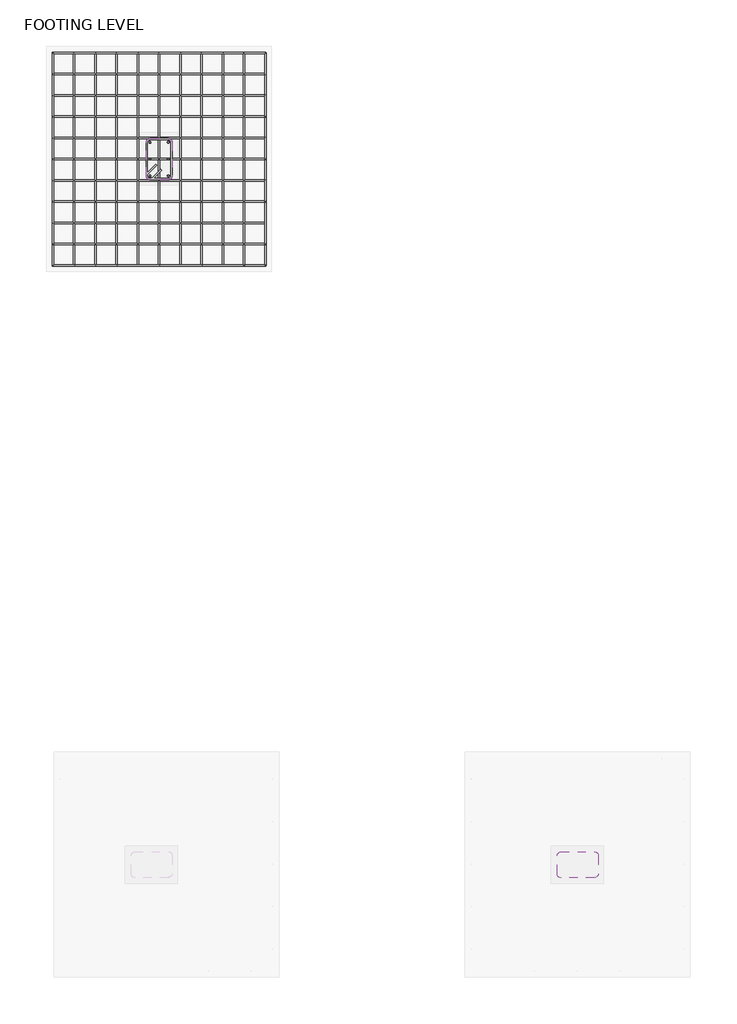
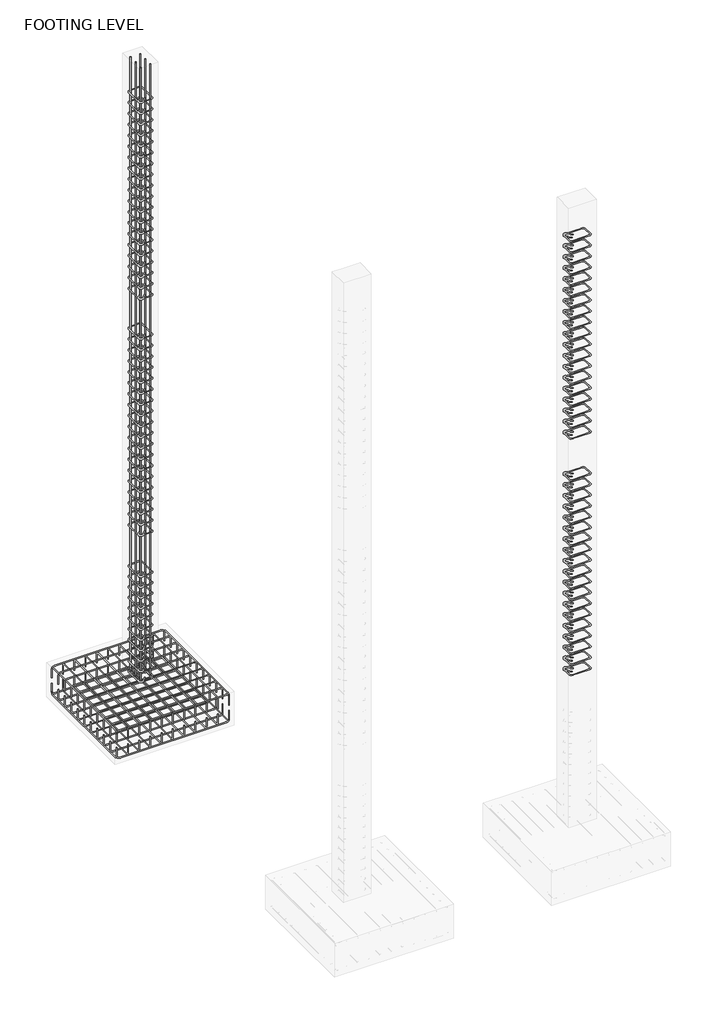
# One storey, part 9 of 9: 15 reinforcing bars.
"""IFC4 building model written with IfcOpenShell, lengths in millimetres."""

from ifc_helpers import new_model, si_unit, point, frame, origin, place, context, project, spatial, polyline, circle_curve, trimmed, segment, composite_curve, source, transform, mapped, element, save
from ifc_brep_helpers import swept_disk

model = new_model("IFC4")

# Units and contexts
model_context = context("Model", 3, world=origin())
ifc_project = project(units=[si_unit("LENGTHUNIT", "METRE", prefix="MILLI")], contexts=[model_context])

# Site, building, storey
site = spatial("IfcSite", under=ifc_project)
building = spatial("IfcBuilding", under=site)
storey = spatial("IfcBuildingStorey", under=building, Name="FOOTING LEVEL", Elevation=-1981.2)

# Reinforcing bars
placement = place(None, origin())
reinforcing_bar_shape = source(origin(), model_context, "Body", "SolidModel", [
    swept_disk(composite_curve([segment(polyline([(-5419.9458659, 13670.9158402, -2171.7), (-5419.9458659, 13670.9158402, -2057.4)]), True, "CONTINUOUS"), segment(trimmed(circle_curve(frame((-5419.9458659, 13637.5783402, -2057.4), z_axis=(1.0, 0.0, 0.0), x_axis=(0.0, 33.337499999999636, 0.0)), 33.3375), [point((-5419.9458659, 13670.9158402, -2057.4))], [point((-5419.9458659, 13637.5783402, -2024.0625))], True, "CARTESIAN"), True, "CONTINUOUS"), segment(polyline([(-5419.9458659, 13637.5783402, -2024.0625), (-5419.9458659, 12265.9783402, -2024.0625)]), True, "CONTINUOUS"), segment(trimmed(circle_curve(frame((-5419.9458659, 12265.9783402, -2057.4), z_axis=(1.0, 0.0, 0.0), x_axis=(0.0, 0.0, 33.33750000000009)), 33.3375), [point((-5419.9458659, 12265.9783402, -2024.0625))], [point((-5419.9458659, 12232.6408402, -2057.4))], True, "CARTESIAN"), True, "CONTINUOUS"), segment(polyline([(-5419.9458659, 12232.6408402, -2057.4), (-5419.9458659, 12232.6408402, -2171.7)]), True, "CONTINUOUS")], self_intersect=False), 4.7625),
])
element("IfcReinforcingBar", 1, at=placement, inside=storey, context=model_context, shape_type="MappedRepresentation", body=[
    mapped(reinforcing_bar_shape, transform((0.0, 0.0, 0.0), x_axis=(1.0, 0.0, 0.0), y_axis=(0.0, 1.0, 0.0), z_axis=(0.0, 0.0, 1.0))),
    mapped(reinforcing_bar_shape, transform((-143.8275, 0.0, 0.0), x_axis=(1.0, 0.0, 0.0), y_axis=(0.0, 1.0, 0.0), z_axis=(0.0, 0.0, 1.0))),
    mapped(reinforcing_bar_shape, transform((-287.655, 0.0, 0.0), x_axis=(1.0, 0.0, 0.0), y_axis=(0.0, 1.0, 0.0), z_axis=(0.0, 0.0, 1.0))),
    mapped(reinforcing_bar_shape, transform((-431.4825, 0.0, 0.0), x_axis=(1.0, 0.0, 0.0), y_axis=(0.0, 1.0, 0.0), z_axis=(0.0, 0.0, 1.0))),
    mapped(reinforcing_bar_shape, transform((-575.31, 0.0, 0.0), x_axis=(1.0, 0.0, 0.0), y_axis=(0.0, 1.0, 0.0), z_axis=(0.0, 0.0, 1.0))),
    mapped(reinforcing_bar_shape, transform((-719.1375, 0.0, 0.0), x_axis=(1.0, 0.0, 0.0), y_axis=(0.0, 1.0, 0.0), z_axis=(0.0, 0.0, 1.0))),
    mapped(reinforcing_bar_shape, transform((-862.965, 0.0, 0.0), x_axis=(1.0, 0.0, 0.0), y_axis=(0.0, 1.0, 0.0), z_axis=(0.0, 0.0, 1.0))),
    mapped(reinforcing_bar_shape, transform((-1006.7925, 0.0, 0.0), x_axis=(1.0, 0.0, 0.0), y_axis=(0.0, 1.0, 0.0), z_axis=(0.0, 0.0, 1.0))),
    mapped(reinforcing_bar_shape, transform((-1150.62, 0.0, 0.0), x_axis=(1.0, 0.0, 0.0), y_axis=(0.0, 1.0, 0.0), z_axis=(0.0, 0.0, 1.0))),
    mapped(reinforcing_bar_shape, transform((-1294.4475, 0.0, 0.0), x_axis=(1.0, 0.0, 0.0), y_axis=(0.0, 1.0, 0.0), z_axis=(0.0, 0.0, 1.0))),
    mapped(reinforcing_bar_shape, transform((-1438.275, 0.0, 0.0), x_axis=(1.0, 0.0, 0.0), y_axis=(0.0, 1.0, 0.0), z_axis=(0.0, 0.0, 1.0))),
])
reinforcing_bar_2_shape = source(origin(), model_context, "Body", "SolidModel", [
    swept_disk(composite_curve([segment(polyline([(-5419.9458659, 12232.6408402, -2247.9), (-5419.9458659, 12232.6408402, -2362.2)]), True, "CONTINUOUS"), segment(trimmed(circle_curve(frame((-5419.9458659, 12265.9783402, -2362.2), z_axis=(1.0, 0.0, 0.0), x_axis=(0.0, -33.337499999999636, 0.0)), 33.3375), [point((-5419.9458659, 12232.6408402, -2362.2))], [point((-5419.9458659, 12265.9783402, -2395.5375))], True, "CARTESIAN"), True, "CONTINUOUS"), segment(polyline([(-5419.9458659, 12265.9783402, -2395.5375), (-5419.9458659, 13637.5783402, -2395.5375)]), True, "CONTINUOUS"), segment(trimmed(circle_curve(frame((-5419.9458659, 13637.5783402, -2362.2), z_axis=(1.0, 0.0, 0.0), x_axis=(0.0, 0.0, -33.33750000000009)), 33.3375), [point((-5419.9458659, 13637.5783402, -2395.5375))], [point((-5419.9458659, 13670.9158402, -2362.2))], True, "CARTESIAN"), True, "CONTINUOUS"), segment(polyline([(-5419.9458659, 13670.9158402, -2362.2), (-5419.9458659, 13670.9158402, -2247.9)]), True, "CONTINUOUS")], self_intersect=False), 4.7625),
])
element("IfcReinforcingBar", 2, at=placement, inside=storey, context=model_context, shape_type="MappedRepresentation", body=[
    mapped(reinforcing_bar_2_shape, transform((0.0, 0.0, 0.0), x_axis=(1.0, 0.0, 0.0), y_axis=(0.0, 1.0, 0.0), z_axis=(0.0, 0.0, 1.0))),
    mapped(reinforcing_bar_2_shape, transform((-143.8275, 0.0, 0.0), x_axis=(1.0, 0.0, 0.0), y_axis=(0.0, 1.0, 0.0), z_axis=(0.0, 0.0, 1.0))),
    mapped(reinforcing_bar_2_shape, transform((-287.655, 0.0, 0.0), x_axis=(1.0, 0.0, 0.0), y_axis=(0.0, 1.0, 0.0), z_axis=(0.0, 0.0, 1.0))),
    mapped(reinforcing_bar_2_shape, transform((-431.4825, 0.0, 0.0), x_axis=(1.0, 0.0, 0.0), y_axis=(0.0, 1.0, 0.0), z_axis=(0.0, 0.0, 1.0))),
    mapped(reinforcing_bar_2_shape, transform((-575.31, 0.0, 0.0), x_axis=(1.0, 0.0, 0.0), y_axis=(0.0, 1.0, 0.0), z_axis=(0.0, 0.0, 1.0))),
    mapped(reinforcing_bar_2_shape, transform((-719.1375, 0.0, 0.0), x_axis=(1.0, 0.0, 0.0), y_axis=(0.0, 1.0, 0.0), z_axis=(0.0, 0.0, 1.0))),
    mapped(reinforcing_bar_2_shape, transform((-862.965, 0.0, 0.0), x_axis=(1.0, 0.0, 0.0), y_axis=(0.0, 1.0, 0.0), z_axis=(0.0, 0.0, 1.0))),
    mapped(reinforcing_bar_2_shape, transform((-1006.7925, 0.0, 0.0), x_axis=(1.0, 0.0, 0.0), y_axis=(0.0, 1.0, 0.0), z_axis=(0.0, 0.0, 1.0))),
    mapped(reinforcing_bar_2_shape, transform((-1150.62, 0.0, 0.0), x_axis=(1.0, 0.0, 0.0), y_axis=(0.0, 1.0, 0.0), z_axis=(0.0, 0.0, 1.0))),
    mapped(reinforcing_bar_2_shape, transform((-1294.4475, 0.0, 0.0), x_axis=(1.0, 0.0, 0.0), y_axis=(0.0, 1.0, 0.0), z_axis=(0.0, 0.0, 1.0))),
    mapped(reinforcing_bar_2_shape, transform((-1438.275, 0.0, 0.0), x_axis=(1.0, 0.0, 0.0), y_axis=(0.0, 1.0, 0.0), z_axis=(0.0, 0.0, 1.0))),
])
reinforcing_bar_3_shape = source(origin(), model_context, "Body", "SolidModel", [
    swept_disk(composite_curve([segment(polyline([(-6858.2208659, 13670.9158402, -2171.7), (-6858.2208659, 13670.9158402, -2057.4)]), True, "CONTINUOUS"), segment(trimmed(circle_curve(frame((-6824.8833659, 13670.9158402, -2057.4), z_axis=(0.0, 1.0, 0.0), x_axis=(-33.337499999999636, 0.0, 0.0)), 33.3375), [point((-6858.2208659, 13670.9158402, -2057.4))], [point((-6824.8833659, 13670.9158402, -2024.0625))], True, "CARTESIAN"), True, "CONTINUOUS"), segment(polyline([(-6824.8833659, 13670.9158402, -2024.0625), (-5453.2833659, 13670.9158402, -2024.0625)]), True, "CONTINUOUS"), segment(trimmed(circle_curve(frame((-5453.2833659, 13670.9158402, -2057.4), z_axis=(0.0, 1.0, 0.0), x_axis=(0.0, 0.0, 33.33750000000009)), 33.3375), [point((-5453.2833659, 13670.9158402, -2024.0625))], [point((-5419.9458659, 13670.9158402, -2057.4))], True, "CARTESIAN"), True, "CONTINUOUS"), segment(polyline([(-5419.9458659, 13670.9158402, -2057.4), (-5419.9458659, 13670.9158402, -2171.7)]), True, "CONTINUOUS")], self_intersect=False), 4.7625),
])
element("IfcReinforcingBar", 3, at=placement, inside=storey, context=model_context, shape_type="MappedRepresentation", body=[
    mapped(reinforcing_bar_3_shape, transform((0.0, 0.0, 0.0), x_axis=(1.0, 0.0, 0.0), y_axis=(0.0, 1.0, 0.0), z_axis=(0.0, 0.0, 1.0))),
    mapped(reinforcing_bar_3_shape, transform((0.0, -143.8275, 0.0), x_axis=(1.0, 0.0, 0.0), y_axis=(0.0, 1.0, 0.0), z_axis=(0.0, 0.0, 1.0))),
    mapped(reinforcing_bar_3_shape, transform((0.0, -287.655, 0.0), x_axis=(1.0, 0.0, 0.0), y_axis=(0.0, 1.0, 0.0), z_axis=(0.0, 0.0, 1.0))),
    mapped(reinforcing_bar_3_shape, transform((0.0, -431.4825, 0.0), x_axis=(1.0, 0.0, 0.0), y_axis=(0.0, 1.0, 0.0), z_axis=(0.0, 0.0, 1.0))),
    mapped(reinforcing_bar_3_shape, transform((0.0, -575.31, 0.0), x_axis=(1.0, 0.0, 0.0), y_axis=(0.0, 1.0, 0.0), z_axis=(0.0, 0.0, 1.0))),
    mapped(reinforcing_bar_3_shape, transform((0.0, -719.1375, 0.0), x_axis=(1.0, 0.0, 0.0), y_axis=(0.0, 1.0, 0.0), z_axis=(0.0, 0.0, 1.0))),
    mapped(reinforcing_bar_3_shape, transform((0.0, -862.965, 0.0), x_axis=(1.0, 0.0, 0.0), y_axis=(0.0, 1.0, 0.0), z_axis=(0.0, 0.0, 1.0))),
    mapped(reinforcing_bar_3_shape, transform((0.0, -1006.7925, 0.0), x_axis=(1.0, 0.0, 0.0), y_axis=(0.0, 1.0, 0.0), z_axis=(0.0, 0.0, 1.0))),
    mapped(reinforcing_bar_3_shape, transform((0.0, -1150.62, 0.0), x_axis=(1.0, 0.0, 0.0), y_axis=(0.0, 1.0, 0.0), z_axis=(0.0, 0.0, 1.0))),
    mapped(reinforcing_bar_3_shape, transform((0.0, -1294.4475, 0.0), x_axis=(1.0, 0.0, 0.0), y_axis=(0.0, 1.0, 0.0), z_axis=(0.0, 0.0, 1.0))),
    mapped(reinforcing_bar_3_shape, transform((0.0, -1438.275, 0.0), x_axis=(1.0, 0.0, 0.0), y_axis=(0.0, 1.0, 0.0), z_axis=(0.0, 0.0, 1.0))),
])
reinforcing_bar_4_shape = source(origin(), model_context, "Body", "SolidModel", [
    swept_disk(composite_curve([segment(polyline([(-6858.2208659, 12232.6408402, -2247.9), (-6858.2208659, 12232.6408402, -2362.2)]), True, "CONTINUOUS"), segment(trimmed(circle_curve(frame((-6824.8833659, 12232.6408402, -2362.2), z_axis=(0.0, -1.0, 0.0), x_axis=(-33.337499999999636, 0.0, 0.0)), 33.3375), [point((-6858.2208659, 12232.6408402, -2362.2))], [point((-6824.8833659, 12232.6408402, -2395.5375))], True, "CARTESIAN"), True, "CONTINUOUS"), segment(polyline([(-6824.8833659, 12232.6408402, -2395.5375), (-5453.2833659, 12232.6408402, -2395.5375)]), True, "CONTINUOUS"), segment(trimmed(circle_curve(frame((-5453.2833659, 12232.6408402, -2362.2), z_axis=(0.0, -1.0, 0.0), x_axis=(0.0, 0.0, -33.33750000000009)), 33.3375), [point((-5453.2833659, 12232.6408402, -2395.5375))], [point((-5419.9458659, 12232.6408402, -2362.2))], True, "CARTESIAN"), True, "CONTINUOUS"), segment(polyline([(-5419.9458659, 12232.6408402, -2362.2), (-5419.9458659, 12232.6408402, -2247.9)]), True, "CONTINUOUS")], self_intersect=False), 4.7625),
])
element("IfcReinforcingBar", 4, at=placement, inside=storey, context=model_context, shape_type="MappedRepresentation", body=[
    mapped(reinforcing_bar_4_shape, transform((0.0, 0.0, 0.0), x_axis=(1.0, 0.0, 0.0), y_axis=(0.0, 1.0, 0.0), z_axis=(0.0, 0.0, 1.0))),
    mapped(reinforcing_bar_4_shape, transform((0.0, 143.8275, 0.0), x_axis=(1.0, 0.0, 0.0), y_axis=(0.0, 1.0, 0.0), z_axis=(0.0, 0.0, 1.0))),
    mapped(reinforcing_bar_4_shape, transform((0.0, 287.655, 0.0), x_axis=(1.0, 0.0, 0.0), y_axis=(0.0, 1.0, 0.0), z_axis=(0.0, 0.0, 1.0))),
    mapped(reinforcing_bar_4_shape, transform((0.0, 431.4825, 0.0), x_axis=(1.0, 0.0, 0.0), y_axis=(0.0, 1.0, 0.0), z_axis=(0.0, 0.0, 1.0))),
    mapped(reinforcing_bar_4_shape, transform((0.0, 575.31, 0.0), x_axis=(1.0, 0.0, 0.0), y_axis=(0.0, 1.0, 0.0), z_axis=(0.0, 0.0, 1.0))),
    mapped(reinforcing_bar_4_shape, transform((0.0, 719.1375, 0.0), x_axis=(1.0, 0.0, 0.0), y_axis=(0.0, 1.0, 0.0), z_axis=(0.0, 0.0, 1.0))),
    mapped(reinforcing_bar_4_shape, transform((0.0, 862.965, 0.0), x_axis=(1.0, 0.0, 0.0), y_axis=(0.0, 1.0, 0.0), z_axis=(0.0, 0.0, 1.0))),
    mapped(reinforcing_bar_4_shape, transform((0.0, 1006.7925, 0.0), x_axis=(1.0, 0.0, 0.0), y_axis=(0.0, 1.0, 0.0), z_axis=(0.0, 0.0, 1.0))),
    mapped(reinforcing_bar_4_shape, transform((0.0, 1150.62, 0.0), x_axis=(1.0, 0.0, 0.0), y_axis=(0.0, 1.0, 0.0), z_axis=(0.0, 0.0, 1.0))),
    mapped(reinforcing_bar_4_shape, transform((0.0, 1294.4475, 0.0), x_axis=(1.0, 0.0, 0.0), y_axis=(0.0, 1.0, 0.0), z_axis=(0.0, 0.0, 1.0))),
    mapped(reinforcing_bar_4_shape, transform((0.0, 1438.275, 0.0), x_axis=(1.0, 0.0, 0.0), y_axis=(0.0, 1.0, 0.0), z_axis=(0.0, 0.0, 1.0))),
])
reinforcing_bar_5_shape = source(origin(), model_context, "Body", "SolidModel", [
    swept_disk(composite_curve([segment(polyline([(-6159.3821491, 12914.3555175, -1938.3375), (-6216.2463461, 12857.4913204, -1938.3375)]), True, "CONTINUOUS"), segment(trimmed(circle_curve(frame((-6199.4083659, 12840.6533402, -1938.3375), z_axis=(0.0, 0.0, 1.0), x_axis=(-16.837980199999947, 16.837980199999947, 0.0)), 23.8125), [point((-6216.2463461, 12857.4913204, -1938.3375))], [point((-6199.4083659, 12816.8408402, -1938.3375))], True, "CARTESIAN"), True, "CONTINUOUS"), segment(polyline([(-6199.4083659, 12816.8408402, -1938.3375), (-6078.7583659, 12816.8408402, -1938.3375)]), True, "CONTINUOUS"), segment(trimmed(circle_curve(frame((-6078.7583659, 12840.6533402, -1938.3375), z_axis=(0.0, 0.0, 1.0), x_axis=(0.0, -23.8125, 0.0)), 23.8125), [point((-6078.7583659, 12816.8408402, -1938.3375))], [point((-6054.9458659, 12840.6533402, -1938.3375))], True, "CARTESIAN"), True, "CONTINUOUS"), segment(polyline([(-6054.9458659, 12840.6533402, -1938.3375), (-6054.9458659, 13062.9033402, -1938.3375)]), True, "CONTINUOUS"), segment(trimmed(circle_curve(frame((-6078.7203098, 13062.9033402, -1939.6832232), z_axis=(-0.056513312022656255, 0.0, 0.9984018457335854), x_axis=(23.774443899999824, 0.0, 1.3457231999998385)), 23.8125), [point((-6054.9458659, 13062.9033402, -1938.3375))], [point((-6078.7203098, 13086.7158402, -1939.6832232))], True, "CARTESIAN"), True, "CONTINUOUS"), segment(polyline([(-6078.7203098, 13086.7158402, -1939.6832232), (-6199.4464219, 13086.7158402, -1946.5167768)]), True, "CONTINUOUS"), segment(trimmed(circle_curve(frame((-6199.4464219, 13062.9033402, -1946.5167768), z_axis=(-0.056513312022656255, 0.0, 0.9984018457335854), x_axis=(0.0, 23.8125, 0.0)), 23.8125), [point((-6199.4464219, 13086.7158402, -1946.5167768))], [point((-6223.2208659, 13062.9033402, -1947.8625))], True, "CARTESIAN"), True, "CONTINUOUS"), segment(polyline([(-6223.2208659, 13062.9033402, -1947.8625), (-6223.2208659, 12840.6533402, -1947.8625)]), True, "CONTINUOUS"), segment(trimmed(circle_curve(frame((-6199.4083659, 12840.6533402, -1947.8625), z_axis=(0.0, 0.0, 1.0), x_axis=(-23.8125, 0.0, 0.0)), 23.8125), [point((-6223.2208659, 12840.6533402, -1947.8625))], [point((-6182.5703857, 12823.81536, -1947.8625))], True, "CARTESIAN"), True, "CONTINUOUS"), segment(polyline([(-6182.5703857, 12823.81536, -1947.8625), (-6125.7061886, 12880.679557, -1947.8625)]), True, "CONTINUOUS")], self_intersect=False), 4.7625),
])
element("IfcReinforcingBar", 5, at=placement, inside=storey, context=model_context, shape_type="MappedRepresentation", body=[
    mapped(reinforcing_bar_5_shape, transform((0.0, 0.0, 0.0), x_axis=(1.0, 0.0, 0.0), y_axis=(0.0, 1.0, 0.0), z_axis=(0.0, 0.0, 1.0))),
    mapped(reinforcing_bar_5_shape, transform((0.0, 0.0, 142.5866456), x_axis=(1.0, 0.0, 0.0), y_axis=(0.0, 1.0, 0.0), z_axis=(0.0, 0.0, 1.0))),
    mapped(reinforcing_bar_5_shape, transform((0.0, 0.0, 285.1732912), x_axis=(1.0, 0.0, 0.0), y_axis=(0.0, 1.0, 0.0), z_axis=(0.0, 0.0, 1.0))),
    mapped(reinforcing_bar_5_shape, transform((0.0, 0.0, 427.7599369), x_axis=(1.0, 0.0, 0.0), y_axis=(0.0, 1.0, 0.0), z_axis=(0.0, 0.0, 1.0))),
    mapped(reinforcing_bar_5_shape, transform((0.0, 0.0, 570.3465825), x_axis=(1.0, 0.0, 0.0), y_axis=(0.0, 1.0, 0.0), z_axis=(0.0, 0.0, 1.0))),
    mapped(reinforcing_bar_5_shape, transform((0.0, 0.0, 712.9332281), x_axis=(1.0, 0.0, 0.0), y_axis=(0.0, 1.0, 0.0), z_axis=(0.0, 0.0, 1.0))),
    mapped(reinforcing_bar_5_shape, transform((0.0, 0.0, 855.5198737), x_axis=(1.0, 0.0, 0.0), y_axis=(0.0, 1.0, 0.0), z_axis=(0.0, 0.0, 1.0))),
    mapped(reinforcing_bar_5_shape, transform((0.0, 0.0, 998.1065193), x_axis=(1.0, 0.0, 0.0), y_axis=(0.0, 1.0, 0.0), z_axis=(0.0, 0.0, 1.0))),
    mapped(reinforcing_bar_5_shape, transform((0.0, 0.0, 1140.6931649), x_axis=(1.0, 0.0, 0.0), y_axis=(0.0, 1.0, 0.0), z_axis=(0.0, 0.0, 1.0))),
    mapped(reinforcing_bar_5_shape, transform((0.0, 0.0, 1283.2798106), x_axis=(1.0, 0.0, 0.0), y_axis=(0.0, 1.0, 0.0), z_axis=(0.0, 0.0, 1.0))),
    mapped(reinforcing_bar_5_shape, transform((0.0, 0.0, 1425.8664562), x_axis=(1.0, 0.0, 0.0), y_axis=(0.0, 1.0, 0.0), z_axis=(0.0, 0.0, 1.0))),
])
element("IfcReinforcingBar", 6, at=placement, inside=storey, context=model_context, shape_type="SolidModel", body=[
    swept_disk(composite_curve([segment(polyline([(-6200.8882737, 13065.2596793, -1943.1), (-6200.8882737, 13065.2596793, 6362.7)]), True, "CONTINUOUS")], self_intersect=False), 6.35),
])
element("IfcReinforcingBar", 7, at=placement, inside=storey, context=model_context, shape_type="SolidModel", body=[
    swept_disk(composite_curve([segment(polyline([(-6077.2784581, 13065.2596793, -1943.1), (-6077.2784581, 13065.2596793, 6362.7)]), True, "CONTINUOUS")], self_intersect=False), 6.35),
])
element("IfcReinforcingBar", 8, at=placement, inside=storey, context=model_context, shape_type="SolidModel", body=[
    swept_disk(composite_curve([segment(polyline([(-6200.8882737, 12838.2970011, -1943.1), (-6200.8882737, 12838.2970011, 6362.7)]), True, "CONTINUOUS")], self_intersect=False), 6.35),
])
element("IfcReinforcingBar", 9, at=placement, inside=storey, context=model_context, shape_type="SolidModel", body=[
    swept_disk(composite_curve([segment(polyline([(-6077.2784581, 12838.2970011, -1943.1), (-6077.2784581, 12838.2970011, 6362.7)]), True, "CONTINUOUS")], self_intersect=False), 6.35),
])
element("IfcReinforcingBar", 10, at=placement, inside=storey, context=model_context, shape_type="SolidModel", body=[
    swept_disk(composite_curve([segment(polyline([(-6200.8882737, 12952.5970011, -1943.1), (-6200.8882737, 12952.5970011, 6362.7)]), True, "CONTINUOUS")], self_intersect=False), 6.35),
])
element("IfcReinforcingBar", 11, at=placement, inside=storey, context=model_context, shape_type="SolidModel", body=[
    swept_disk(composite_curve([segment(polyline([(-6077.2784581, 12952.5970011, -1943.1), (-6077.2784581, 12952.5970011, 6362.7)]), True, "CONTINUOUS")], self_intersect=False), 6.35),
])
reinforcing_bar_6_shape = source(origin(), model_context, "Body", "SolidModel", [
    swept_disk(composite_curve([segment(polyline([(-6159.3821491, 12914.3555175, 42.8625), (-6216.2463461, 12857.4913204, 42.8625)]), True, "CONTINUOUS"), segment(trimmed(circle_curve(frame((-6199.4083659, 12840.6533402, 42.8625), z_axis=(0.0, 0.0, 1.0), x_axis=(-16.837980199999947, 16.837980199999947, 0.0)), 23.8125), [point((-6216.2463461, 12857.4913204, 42.8625))], [point((-6199.4083659, 12816.8408402, 42.8625))], True, "CARTESIAN"), True, "CONTINUOUS"), segment(polyline([(-6199.4083659, 12816.8408402, 42.8625), (-6078.7583659, 12816.8408402, 42.8625)]), True, "CONTINUOUS"), segment(trimmed(circle_curve(frame((-6078.7583659, 12840.6533402, 42.8625), z_axis=(0.0, 0.0, 1.0), x_axis=(0.0, -23.8125, 0.0)), 23.8125), [point((-6078.7583659, 12816.8408402, 42.8625))], [point((-6054.9458659, 12840.6533402, 42.8625))], True, "CARTESIAN"), True, "CONTINUOUS"), segment(polyline([(-6054.9458659, 12840.6533402, 42.8625), (-6054.9458659, 13062.9033402, 42.8625)]), True, "CONTINUOUS"), segment(trimmed(circle_curve(frame((-6078.7203098, 13062.9033402, 41.5167768), z_axis=(-0.056513312022656255, 0.0, 0.9984018457335854), x_axis=(23.774443899999824, 0.0, 1.3457231999999948)), 23.8125), [point((-6054.9458659, 13062.9033402, 42.8625))], [point((-6078.7203098, 13086.7158402, 41.5167768))], True, "CARTESIAN"), True, "CONTINUOUS"), segment(polyline([(-6078.7203098, 13086.7158402, 41.5167768), (-6199.4464219, 13086.7158402, 34.6832232)]), True, "CONTINUOUS"), segment(trimmed(circle_curve(frame((-6199.4464219, 13062.9033402, 34.6832232), z_axis=(-0.056513312022656255, 0.0, 0.9984018457335854), x_axis=(0.0, 23.8125, 0.0)), 23.8125), [point((-6199.4464219, 13086.7158402, 34.6832232))], [point((-6223.2208659, 13062.9033402, 33.3375))], True, "CARTESIAN"), True, "CONTINUOUS"), segment(polyline([(-6223.2208659, 13062.9033402, 33.3375), (-6223.2208659, 12840.6533402, 33.3375)]), True, "CONTINUOUS"), segment(trimmed(circle_curve(frame((-6199.4083659, 12840.6533402, 33.3375), z_axis=(0.0, 0.0, 1.0), x_axis=(-23.8125, 0.0, 0.0)), 23.8125), [point((-6223.2208659, 12840.6533402, 33.3375))], [point((-6182.5703857, 12823.81536, 33.3375))], True, "CARTESIAN"), True, "CONTINUOUS"), segment(polyline([(-6182.5703857, 12823.81536, 33.3375), (-6125.7061886, 12880.679557, 33.3375)]), True, "CONTINUOUS")], self_intersect=False), 4.7625),
])
element("IfcReinforcingBar", 12, at=placement, inside=storey, context=model_context, shape_type="MappedRepresentation", body=[
    mapped(reinforcing_bar_6_shape, transform((0.0, 0.0, 0.0), x_axis=(1.0, 0.0, 0.0), y_axis=(0.0, 1.0, 0.0), z_axis=(0.0, 0.0, 1.0))),
    mapped(reinforcing_bar_6_shape, transform((0.0, 0.0, 147.8567446), x_axis=(1.0, 0.0, 0.0), y_axis=(0.0, 1.0, 0.0), z_axis=(0.0, 0.0, 1.0))),
    mapped(reinforcing_bar_6_shape, transform((0.0, 0.0, 295.7134892), x_axis=(1.0, 0.0, 0.0), y_axis=(0.0, 1.0, 0.0), z_axis=(0.0, 0.0, 1.0))),
    mapped(reinforcing_bar_6_shape, transform((0.0, 0.0, 443.5702338), x_axis=(1.0, 0.0, 0.0), y_axis=(0.0, 1.0, 0.0), z_axis=(0.0, 0.0, 1.0))),
    mapped(reinforcing_bar_6_shape, transform((0.0, 0.0, 591.4269784), x_axis=(1.0, 0.0, 0.0), y_axis=(0.0, 1.0, 0.0), z_axis=(0.0, 0.0, 1.0))),
    mapped(reinforcing_bar_6_shape, transform((0.0, 0.0, 739.283723), x_axis=(1.0, 0.0, 0.0), y_axis=(0.0, 1.0, 0.0), z_axis=(0.0, 0.0, 1.0))),
    mapped(reinforcing_bar_6_shape, transform((0.0, 0.0, 887.1404675), x_axis=(1.0, 0.0, 0.0), y_axis=(0.0, 1.0, 0.0), z_axis=(0.0, 0.0, 1.0))),
    mapped(reinforcing_bar_6_shape, transform((0.0, 0.0, 1034.9972121), x_axis=(1.0, 0.0, 0.0), y_axis=(0.0, 1.0, 0.0), z_axis=(0.0, 0.0, 1.0))),
    mapped(reinforcing_bar_6_shape, transform((0.0, 0.0, 1182.8539567), x_axis=(1.0, 0.0, 0.0), y_axis=(0.0, 1.0, 0.0), z_axis=(0.0, 0.0, 1.0))),
    mapped(reinforcing_bar_6_shape, transform((0.0, 0.0, 1330.7107013), x_axis=(1.0, 0.0, 0.0), y_axis=(0.0, 1.0, 0.0), z_axis=(0.0, 0.0, 1.0))),
    mapped(reinforcing_bar_6_shape, transform((0.0, 0.0, 1478.5674459), x_axis=(1.0, 0.0, 0.0), y_axis=(0.0, 1.0, 0.0), z_axis=(0.0, 0.0, 1.0))),
    mapped(reinforcing_bar_6_shape, transform((0.0, 0.0, 1626.4241905), x_axis=(1.0, 0.0, 0.0), y_axis=(0.0, 1.0, 0.0), z_axis=(0.0, 0.0, 1.0))),
    mapped(reinforcing_bar_6_shape, transform((0.0, 0.0, 1774.2809351), x_axis=(1.0, 0.0, 0.0), y_axis=(0.0, 1.0, 0.0), z_axis=(0.0, 0.0, 1.0))),
    mapped(reinforcing_bar_6_shape, transform((0.0, 0.0, 1922.1376797), x_axis=(1.0, 0.0, 0.0), y_axis=(0.0, 1.0, 0.0), z_axis=(0.0, 0.0, 1.0))),
    mapped(reinforcing_bar_6_shape, transform((0.0, 0.0, 2069.9944243), x_axis=(1.0, 0.0, 0.0), y_axis=(0.0, 1.0, 0.0), z_axis=(0.0, 0.0, 1.0))),
    mapped(reinforcing_bar_6_shape, transform((0.0, 0.0, 2217.8511689), x_axis=(1.0, 0.0, 0.0), y_axis=(0.0, 1.0, 0.0), z_axis=(0.0, 0.0, 1.0))),
    mapped(reinforcing_bar_6_shape, transform((0.0, 0.0, 2365.7079134), x_axis=(1.0, 0.0, 0.0), y_axis=(0.0, 1.0, 0.0), z_axis=(0.0, 0.0, 1.0))),
    mapped(reinforcing_bar_6_shape, transform((0.0, 0.0, 2513.564658), x_axis=(1.0, 0.0, 0.0), y_axis=(0.0, 1.0, 0.0), z_axis=(0.0, 0.0, 1.0))),
    mapped(reinforcing_bar_6_shape, transform((0.0, 0.0, 2661.4214026), x_axis=(1.0, 0.0, 0.0), y_axis=(0.0, 1.0, 0.0), z_axis=(0.0, 0.0, 1.0))),
])
reinforcing_bar_7_shape = source(origin(), model_context, "Body", "SolidModel", [
    swept_disk(composite_curve([segment(polyline([(-6159.3821491, 12914.3555175, 3243.2625), (-6216.2463461, 12857.4913204, 3243.2625)]), True, "CONTINUOUS"), segment(trimmed(circle_curve(frame((-6199.4083659, 12840.6533402, 3243.2625), z_axis=(0.0, 0.0, 1.0), x_axis=(-16.837980199999947, 16.837980199999947, 0.0)), 23.8125), [point((-6216.2463461, 12857.4913204, 3243.2625))], [point((-6199.4083659, 12816.8408402, 3243.2625))], True, "CARTESIAN"), True, "CONTINUOUS"), segment(polyline([(-6199.4083659, 12816.8408402, 3243.2625), (-6078.7583659, 12816.8408402, 3243.2625)]), True, "CONTINUOUS"), segment(trimmed(circle_curve(frame((-6078.7583659, 12840.6533402, 3243.2625), z_axis=(0.0, 0.0, 1.0), x_axis=(0.0, -23.8125, 0.0)), 23.8125), [point((-6078.7583659, 12816.8408402, 3243.2625))], [point((-6054.9458659, 12840.6533402, 3243.2625))], True, "CARTESIAN"), True, "CONTINUOUS"), segment(polyline([(-6054.9458659, 12840.6533402, 3243.2625), (-6054.9458659, 13062.9033402, 3243.2625)]), True, "CONTINUOUS"), segment(trimmed(circle_curve(frame((-6078.7203098, 13062.9033402, 3241.9167768), z_axis=(-0.056513312022656255, 0.0, 0.9984018457335854), x_axis=(23.774443899999824, 0.0, 1.345723199999611)), 23.8125), [point((-6054.9458659, 13062.9033402, 3243.2625))], [point((-6078.7203098, 13086.7158402, 3241.9167768))], True, "CARTESIAN"), True, "CONTINUOUS"), segment(polyline([(-6078.7203098, 13086.7158402, 3241.9167768), (-6199.4464219, 13086.7158402, 3235.0832232)]), True, "CONTINUOUS"), segment(trimmed(circle_curve(frame((-6199.4464219, 13062.9033402, 3235.0832232), z_axis=(-0.056513312022656255, 0.0, 0.9984018457335854), x_axis=(0.0, 23.8125, 0.0)), 23.8125), [point((-6199.4464219, 13086.7158402, 3235.0832232))], [point((-6223.2208659, 13062.9033402, 3233.7375))], True, "CARTESIAN"), True, "CONTINUOUS"), segment(polyline([(-6223.2208659, 13062.9033402, 3233.7375), (-6223.2208659, 12840.6533402, 3233.7375)]), True, "CONTINUOUS"), segment(trimmed(circle_curve(frame((-6199.4083659, 12840.6533402, 3233.7375), z_axis=(0.0, 0.0, 1.0), x_axis=(-23.8125, 0.0, 0.0)), 23.8125), [point((-6223.2208659, 12840.6533402, 3233.7375))], [point((-6182.5703857, 12823.81536, 3233.7375))], True, "CARTESIAN"), True, "CONTINUOUS"), segment(polyline([(-6182.5703857, 12823.81536, 3233.7375), (-6125.7061886, 12880.679557, 3233.7375)]), True, "CONTINUOUS")], self_intersect=False), 4.7625),
])
element("IfcReinforcingBar", 13, at=placement, inside=storey, context=model_context, shape_type="MappedRepresentation", body=[
    mapped(reinforcing_bar_7_shape, transform((0.0, 0.0, 0.0), x_axis=(1.0, 0.0, 0.0), y_axis=(0.0, 1.0, 0.0), z_axis=(0.0, 0.0, 1.0))),
    mapped(reinforcing_bar_7_shape, transform((0.0, 0.0, 147.8770493), x_axis=(1.0, 0.0, 0.0), y_axis=(0.0, 1.0, 0.0), z_axis=(0.0, 0.0, 1.0))),
    mapped(reinforcing_bar_7_shape, transform((0.0, 0.0, 295.7540986), x_axis=(1.0, 0.0, 0.0), y_axis=(0.0, 1.0, 0.0), z_axis=(0.0, 0.0, 1.0))),
    mapped(reinforcing_bar_7_shape, transform((0.0, 0.0, 443.6311479), x_axis=(1.0, 0.0, 0.0), y_axis=(0.0, 1.0, 0.0), z_axis=(0.0, 0.0, 1.0))),
    mapped(reinforcing_bar_7_shape, transform((0.0, 0.0, 591.5081972), x_axis=(1.0, 0.0, 0.0), y_axis=(0.0, 1.0, 0.0), z_axis=(0.0, 0.0, 1.0))),
    mapped(reinforcing_bar_7_shape, transform((0.0, 0.0, 739.3852464), x_axis=(1.0, 0.0, 0.0), y_axis=(0.0, 1.0, 0.0), z_axis=(0.0, 0.0, 1.0))),
    mapped(reinforcing_bar_7_shape, transform((0.0, 0.0, 887.2622957), x_axis=(1.0, 0.0, 0.0), y_axis=(0.0, 1.0, 0.0), z_axis=(0.0, 0.0, 1.0))),
    mapped(reinforcing_bar_7_shape, transform((0.0, 0.0, 1035.139345), x_axis=(1.0, 0.0, 0.0), y_axis=(0.0, 1.0, 0.0), z_axis=(0.0, 0.0, 1.0))),
    mapped(reinforcing_bar_7_shape, transform((0.0, 0.0, 1183.0163943), x_axis=(1.0, 0.0, 0.0), y_axis=(0.0, 1.0, 0.0), z_axis=(0.0, 0.0, 1.0))),
    mapped(reinforcing_bar_7_shape, transform((0.0, 0.0, 1330.8934436), x_axis=(1.0, 0.0, 0.0), y_axis=(0.0, 1.0, 0.0), z_axis=(0.0, 0.0, 1.0))),
    mapped(reinforcing_bar_7_shape, transform((0.0, 0.0, 1478.7704929), x_axis=(1.0, 0.0, 0.0), y_axis=(0.0, 1.0, 0.0), z_axis=(0.0, 0.0, 1.0))),
    mapped(reinforcing_bar_7_shape, transform((0.0, 0.0, 1626.6475422), x_axis=(1.0, 0.0, 0.0), y_axis=(0.0, 1.0, 0.0), z_axis=(0.0, 0.0, 1.0))),
    mapped(reinforcing_bar_7_shape, transform((0.0, 0.0, 1774.5245915), x_axis=(1.0, 0.0, 0.0), y_axis=(0.0, 1.0, 0.0), z_axis=(0.0, 0.0, 1.0))),
    mapped(reinforcing_bar_7_shape, transform((0.0, 0.0, 1922.4016408), x_axis=(1.0, 0.0, 0.0), y_axis=(0.0, 1.0, 0.0), z_axis=(0.0, 0.0, 1.0))),
    mapped(reinforcing_bar_7_shape, transform((0.0, 0.0, 2070.2786901), x_axis=(1.0, 0.0, 0.0), y_axis=(0.0, 1.0, 0.0), z_axis=(0.0, 0.0, 1.0))),
    mapped(reinforcing_bar_7_shape, transform((0.0, 0.0, 2218.1557393), x_axis=(1.0, 0.0, 0.0), y_axis=(0.0, 1.0, 0.0), z_axis=(0.0, 0.0, 1.0))),
    mapped(reinforcing_bar_7_shape, transform((0.0, 0.0, 2366.0327886), x_axis=(1.0, 0.0, 0.0), y_axis=(0.0, 1.0, 0.0), z_axis=(0.0, 0.0, 1.0))),
    mapped(reinforcing_bar_7_shape, transform((0.0, 0.0, 2513.9098379), x_axis=(1.0, 0.0, 0.0), y_axis=(0.0, 1.0, 0.0), z_axis=(0.0, 0.0, 1.0))),
    mapped(reinforcing_bar_7_shape, transform((0.0, 0.0, 2661.7868872), x_axis=(1.0, 0.0, 0.0), y_axis=(0.0, 1.0, 0.0), z_axis=(0.0, 0.0, 1.0))),
])
reinforcing_bar_8_shape = source(origin(), model_context, "Body", "SolidModel", [
    swept_disk(composite_curve([segment(polyline([(-3344.4061886, 8196.8771233, 42.8625), (-3401.2703857, 8253.7413204, 42.8625)]), True, "CONTINUOUS"), segment(trimmed(circle_curve(frame((-3418.1083659, 8236.9033402, 42.8625), z_axis=(0.0, 0.0, 1.0), x_axis=(16.837980199999947, 16.837980199999947, 0.0)), 23.8125), [point((-3401.2703857, 8253.7413204, 42.8625))], [point((-3441.9208659, 8236.9033402, 42.8625))], True, "CARTESIAN"), True, "CONTINUOUS"), segment(polyline([(-3441.9208659, 8236.9033402, 42.8625), (-3441.9208659, 8116.2533402, 42.8625)]), True, "CONTINUOUS"), segment(trimmed(circle_curve(frame((-3418.1083659, 8116.2533402, 42.8625), z_axis=(0.0, 0.0, 1.0), x_axis=(-23.8125, 0.0, 0.0)), 23.8125), [point((-3441.9208659, 8116.2533402, 42.8625))], [point((-3418.1083659, 8092.4408402, 42.8625))], True, "CARTESIAN"), True, "CONTINUOUS"), segment(polyline([(-3418.1083659, 8092.4408402, 42.8625), (-3195.8583659, 8092.4408402, 42.8625)]), True, "CONTINUOUS"), segment(trimmed(circle_curve(frame((-3195.8583659, 8116.2152841, 41.5167768), z_axis=(0.0, 0.056513312022656255, 0.9984018457335854), x_axis=(0.0, -23.774443899999824, 1.3457231999999948)), 23.8125), [point((-3195.8583659, 8092.4408402, 42.8625))], [point((-3172.0458659, 8116.2152841, 41.5167768))], True, "CARTESIAN"), True, "CONTINUOUS"), segment(polyline([(-3172.0458659, 8116.2152841, 41.5167768), (-3172.0458659, 8236.9413962, 34.6832232)]), True, "CONTINUOUS"), segment(trimmed(circle_curve(frame((-3195.8583659, 8236.9413962, 34.6832232), z_axis=(0.0, 0.056513312022656255, 0.9984018457335854), x_axis=(23.8125, 0.0, 0.0)), 23.8125), [point((-3172.0458659, 8236.9413962, 34.6832232))], [point((-3195.8583659, 8260.7158402, 33.3375))], True, "CARTESIAN"), True, "CONTINUOUS"), segment(polyline([(-3195.8583659, 8260.7158402, 33.3375), (-3418.1083659, 8260.7158402, 33.3375)]), True, "CONTINUOUS"), segment(trimmed(circle_curve(frame((-3418.1083659, 8236.9033402, 33.3375), z_axis=(0.0, 0.0, 1.0), x_axis=(0.0, 23.8125, 0.0)), 23.8125), [point((-3418.1083659, 8260.7158402, 33.3375))], [point((-3434.9463461, 8220.06536, 33.3375))], True, "CARTESIAN"), True, "CONTINUOUS"), segment(polyline([(-3434.9463461, 8220.06536, 33.3375), (-3378.0821491, 8163.2011629, 33.3375)]), True, "CONTINUOUS")], self_intersect=False), 4.7625),
])
element("IfcReinforcingBar", 14, at=placement, inside=storey, context=model_context, shape_type="MappedRepresentation", body=[
    mapped(reinforcing_bar_8_shape, transform((0.0, 0.0, 0.0), x_axis=(1.0, 0.0, 0.0), y_axis=(0.0, 1.0, 0.0), z_axis=(0.0, 0.0, 1.0))),
    mapped(reinforcing_bar_8_shape, transform((0.0, 0.0, 146.5540169), x_axis=(1.0, 0.0, 0.0), y_axis=(0.0, 1.0, 0.0), z_axis=(0.0, 0.0, 1.0))),
    mapped(reinforcing_bar_8_shape, transform((0.0, 0.0, 293.1080338), x_axis=(1.0, 0.0, 0.0), y_axis=(0.0, 1.0, 0.0), z_axis=(0.0, 0.0, 1.0))),
    mapped(reinforcing_bar_8_shape, transform((0.0, 0.0, 439.6620507), x_axis=(1.0, 0.0, 0.0), y_axis=(0.0, 1.0, 0.0), z_axis=(0.0, 0.0, 1.0))),
    mapped(reinforcing_bar_8_shape, transform((0.0, 0.0, 586.2160676), x_axis=(1.0, 0.0, 0.0), y_axis=(0.0, 1.0, 0.0), z_axis=(0.0, 0.0, 1.0))),
    mapped(reinforcing_bar_8_shape, transform((0.0, 0.0, 732.7700846), x_axis=(1.0, 0.0, 0.0), y_axis=(0.0, 1.0, 0.0), z_axis=(0.0, 0.0, 1.0))),
    mapped(reinforcing_bar_8_shape, transform((0.0, 0.0, 879.3241015), x_axis=(1.0, 0.0, 0.0), y_axis=(0.0, 1.0, 0.0), z_axis=(0.0, 0.0, 1.0))),
    mapped(reinforcing_bar_8_shape, transform((0.0, 0.0, 1025.8781184), x_axis=(1.0, 0.0, 0.0), y_axis=(0.0, 1.0, 0.0), z_axis=(0.0, 0.0, 1.0))),
    mapped(reinforcing_bar_8_shape, transform((0.0, 0.0, 1172.4321353), x_axis=(1.0, 0.0, 0.0), y_axis=(0.0, 1.0, 0.0), z_axis=(0.0, 0.0, 1.0))),
    mapped(reinforcing_bar_8_shape, transform((0.0, 0.0, 1318.9861522), x_axis=(1.0, 0.0, 0.0), y_axis=(0.0, 1.0, 0.0), z_axis=(0.0, 0.0, 1.0))),
    mapped(reinforcing_bar_8_shape, transform((0.0, 0.0, 1465.5401691), x_axis=(1.0, 0.0, 0.0), y_axis=(0.0, 1.0, 0.0), z_axis=(0.0, 0.0, 1.0))),
    mapped(reinforcing_bar_8_shape, transform((0.0, 0.0, 1612.094186), x_axis=(1.0, 0.0, 0.0), y_axis=(0.0, 1.0, 0.0), z_axis=(0.0, 0.0, 1.0))),
    mapped(reinforcing_bar_8_shape, transform((0.0, 0.0, 1758.6482029), x_axis=(1.0, 0.0, 0.0), y_axis=(0.0, 1.0, 0.0), z_axis=(0.0, 0.0, 1.0))),
    mapped(reinforcing_bar_8_shape, transform((0.0, 0.0, 1905.2022198), x_axis=(1.0, 0.0, 0.0), y_axis=(0.0, 1.0, 0.0), z_axis=(0.0, 0.0, 1.0))),
    mapped(reinforcing_bar_8_shape, transform((0.0, 0.0, 2051.7562368), x_axis=(1.0, 0.0, 0.0), y_axis=(0.0, 1.0, 0.0), z_axis=(0.0, 0.0, 1.0))),
    mapped(reinforcing_bar_8_shape, transform((0.0, 0.0, 2198.3102537), x_axis=(1.0, 0.0, 0.0), y_axis=(0.0, 1.0, 0.0), z_axis=(0.0, 0.0, 1.0))),
    mapped(reinforcing_bar_8_shape, transform((0.0, 0.0, 2344.8642706), x_axis=(1.0, 0.0, 0.0), y_axis=(0.0, 1.0, 0.0), z_axis=(0.0, 0.0, 1.0))),
    mapped(reinforcing_bar_8_shape, transform((0.0, 0.0, 2491.4182875), x_axis=(1.0, 0.0, 0.0), y_axis=(0.0, 1.0, 0.0), z_axis=(0.0, 0.0, 1.0))),
    mapped(reinforcing_bar_8_shape, transform((0.0, 0.0, 2637.9723044), x_axis=(1.0, 0.0, 0.0), y_axis=(0.0, 1.0, 0.0), z_axis=(0.0, 0.0, 1.0))),
])
reinforcing_bar_9_shape = source(origin(), model_context, "Body", "SolidModel", [
    swept_disk(composite_curve([segment(polyline([(-3344.4061886, 8196.8771233, 3243.2625), (-3401.2703857, 8253.7413204, 3243.2625)]), True, "CONTINUOUS"), segment(trimmed(circle_curve(frame((-3418.1083659, 8236.9033402, 3243.2625), z_axis=(0.0, 0.0, 1.0), x_axis=(16.837980199999947, 16.837980199999947, 0.0)), 23.8125), [point((-3401.2703857, 8253.7413204, 3243.2625))], [point((-3441.9208659, 8236.9033402, 3243.2625))], True, "CARTESIAN"), True, "CONTINUOUS"), segment(polyline([(-3441.9208659, 8236.9033402, 3243.2625), (-3441.9208659, 8116.2533402, 3243.2625)]), True, "CONTINUOUS"), segment(trimmed(circle_curve(frame((-3418.1083659, 8116.2533402, 3243.2625), z_axis=(0.0, 0.0, 1.0), x_axis=(-23.8125, 0.0, 0.0)), 23.8125), [point((-3441.9208659, 8116.2533402, 3243.2625))], [point((-3418.1083659, 8092.4408402, 3243.2625))], True, "CARTESIAN"), True, "CONTINUOUS"), segment(polyline([(-3418.1083659, 8092.4408402, 3243.2625), (-3195.8583659, 8092.4408402, 3243.2625)]), True, "CONTINUOUS"), segment(trimmed(circle_curve(frame((-3195.8583659, 8116.2152841, 3241.9167768), z_axis=(0.0, 0.056513312022656255, 0.9984018457335854), x_axis=(0.0, -23.774443899999824, 1.345723199999611)), 23.8125), [point((-3195.8583659, 8092.4408402, 3243.2625))], [point((-3172.0458659, 8116.2152841, 3241.9167768))], True, "CARTESIAN"), True, "CONTINUOUS"), segment(polyline([(-3172.0458659, 8116.2152841, 3241.9167768), (-3172.0458659, 8236.9413962, 3235.0832232)]), True, "CONTINUOUS"), segment(trimmed(circle_curve(frame((-3195.8583659, 8236.9413962, 3235.0832232), z_axis=(0.0, 0.056513312022656255, 0.9984018457335854), x_axis=(23.8125, 0.0, 0.0)), 23.8125), [point((-3172.0458659, 8236.9413962, 3235.0832232))], [point((-3195.8583659, 8260.7158402, 3233.7375))], True, "CARTESIAN"), True, "CONTINUOUS"), segment(polyline([(-3195.8583659, 8260.7158402, 3233.7375), (-3418.1083659, 8260.7158402, 3233.7375)]), True, "CONTINUOUS"), segment(trimmed(circle_curve(frame((-3418.1083659, 8236.9033402, 3233.7375), z_axis=(0.0, 0.0, 1.0), x_axis=(0.0, 23.8125, 0.0)), 23.8125), [point((-3418.1083659, 8260.7158402, 3233.7375))], [point((-3434.9463461, 8220.06536, 3233.7375))], True, "CARTESIAN"), True, "CONTINUOUS"), segment(polyline([(-3434.9463461, 8220.06536, 3233.7375), (-3378.0821491, 8163.2011629, 3233.7375)]), True, "CONTINUOUS")], self_intersect=False), 4.7625),
])
element("IfcReinforcingBar", 15, at=placement, inside=storey, context=model_context, shape_type="MappedRepresentation", body=[
    mapped(reinforcing_bar_9_shape, transform((0.0, 0.0, 0.0), x_axis=(1.0, 0.0, 0.0), y_axis=(0.0, 1.0, 0.0), z_axis=(0.0, 0.0, 1.0))),
    mapped(reinforcing_bar_9_shape, transform((0.0, 0.0, 148.4372585), x_axis=(1.0, 0.0, 0.0), y_axis=(0.0, 1.0, 0.0), z_axis=(0.0, 0.0, 1.0))),
    mapped(reinforcing_bar_9_shape, transform((0.0, 0.0, 296.8745169), x_axis=(1.0, 0.0, 0.0), y_axis=(0.0, 1.0, 0.0), z_axis=(0.0, 0.0, 1.0))),
    mapped(reinforcing_bar_9_shape, transform((0.0, 0.0, 445.3117754), x_axis=(1.0, 0.0, 0.0), y_axis=(0.0, 1.0, 0.0), z_axis=(0.0, 0.0, 1.0))),
    mapped(reinforcing_bar_9_shape, transform((0.0, 0.0, 593.7490338), x_axis=(1.0, 0.0, 0.0), y_axis=(0.0, 1.0, 0.0), z_axis=(0.0, 0.0, 1.0))),
    mapped(reinforcing_bar_9_shape, transform((0.0, 0.0, 742.1862923), x_axis=(1.0, 0.0, 0.0), y_axis=(0.0, 1.0, 0.0), z_axis=(0.0, 0.0, 1.0))),
    mapped(reinforcing_bar_9_shape, transform((0.0, 0.0, 890.6235507), x_axis=(1.0, 0.0, 0.0), y_axis=(0.0, 1.0, 0.0), z_axis=(0.0, 0.0, 1.0))),
    mapped(reinforcing_bar_9_shape, transform((0.0, 0.0, 1039.0608092), x_axis=(1.0, 0.0, 0.0), y_axis=(0.0, 1.0, 0.0), z_axis=(0.0, 0.0, 1.0))),
    mapped(reinforcing_bar_9_shape, transform((0.0, 0.0, 1187.4980677), x_axis=(1.0, 0.0, 0.0), y_axis=(0.0, 1.0, 0.0), z_axis=(0.0, 0.0, 1.0))),
    mapped(reinforcing_bar_9_shape, transform((0.0, 0.0, 1335.9353261), x_axis=(1.0, 0.0, 0.0), y_axis=(0.0, 1.0, 0.0), z_axis=(0.0, 0.0, 1.0))),
    mapped(reinforcing_bar_9_shape, transform((0.0, 0.0, 1484.3725846), x_axis=(1.0, 0.0, 0.0), y_axis=(0.0, 1.0, 0.0), z_axis=(0.0, 0.0, 1.0))),
    mapped(reinforcing_bar_9_shape, transform((0.0, 0.0, 1632.809843), x_axis=(1.0, 0.0, 0.0), y_axis=(0.0, 1.0, 0.0), z_axis=(0.0, 0.0, 1.0))),
    mapped(reinforcing_bar_9_shape, transform((0.0, 0.0, 1781.2471015), x_axis=(1.0, 0.0, 0.0), y_axis=(0.0, 1.0, 0.0), z_axis=(0.0, 0.0, 1.0))),
    mapped(reinforcing_bar_9_shape, transform((0.0, 0.0, 1929.6843599), x_axis=(1.0, 0.0, 0.0), y_axis=(0.0, 1.0, 0.0), z_axis=(0.0, 0.0, 1.0))),
    mapped(reinforcing_bar_9_shape, transform((0.0, 0.0, 2078.1216184), x_axis=(1.0, 0.0, 0.0), y_axis=(0.0, 1.0, 0.0), z_axis=(0.0, 0.0, 1.0))),
    mapped(reinforcing_bar_9_shape, transform((0.0, 0.0, 2226.5588768), x_axis=(1.0, 0.0, 0.0), y_axis=(0.0, 1.0, 0.0), z_axis=(0.0, 0.0, 1.0))),
    mapped(reinforcing_bar_9_shape, transform((0.0, 0.0, 2374.9961353), x_axis=(1.0, 0.0, 0.0), y_axis=(0.0, 1.0, 0.0), z_axis=(0.0, 0.0, 1.0))),
    mapped(reinforcing_bar_9_shape, transform((0.0, 0.0, 2523.4333938), x_axis=(1.0, 0.0, 0.0), y_axis=(0.0, 1.0, 0.0), z_axis=(0.0, 0.0, 1.0))),
    mapped(reinforcing_bar_9_shape, transform((0.0, 0.0, 2671.8706522), x_axis=(1.0, 0.0, 0.0), y_axis=(0.0, 1.0, 0.0), z_axis=(0.0, 0.0, 1.0))),
])

save(model, "model.ifc")

# Revit data of these elements
# Elements 1, 2, 3, 4, 5, 6, 7, 8, 9, 10, 11, 12, 13, 14, 15 (IfcReinforcingBar)
#   Phase Created = New Construction
